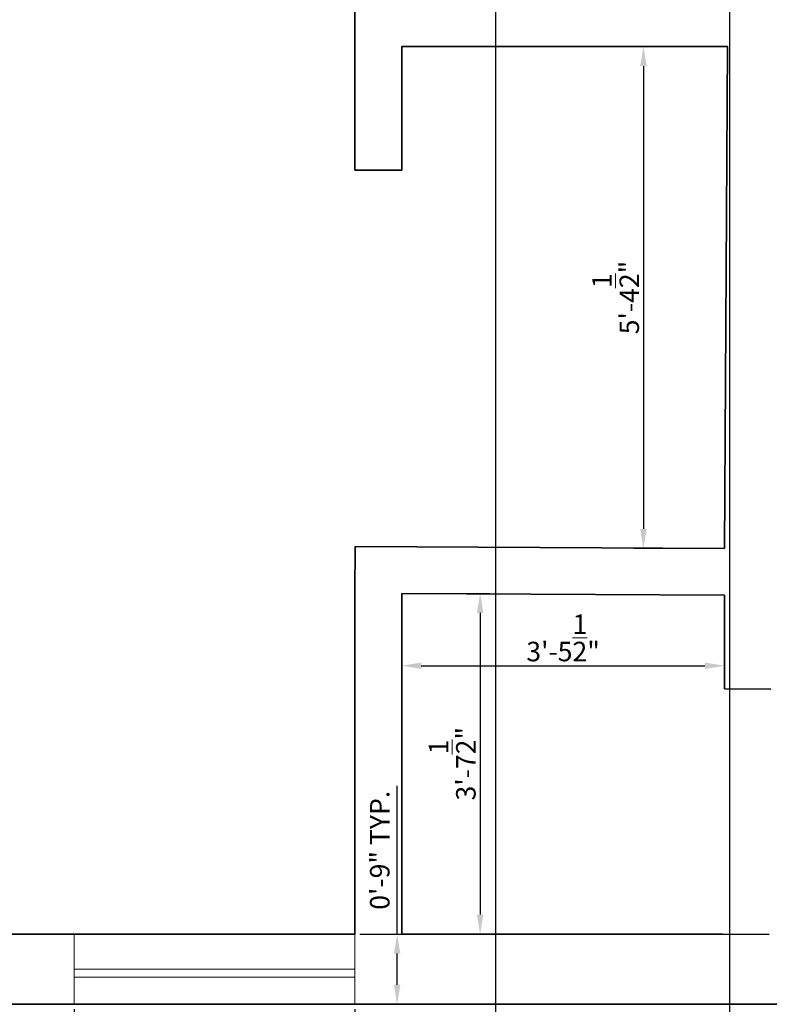
# Model space of a CAD drawing. Units: inches. Extents: x 2025 to 2528, y 1525 to 2336.
# Tile 3 of 18: x 2164 to 2260, y 1704 to 1831. Entities that reach past the tile are written whole.
import ezdxf

# ---------------------------------------------------------------- set-up
doc = ezdxf.new("R2010")
doc.units = ezdxf.units.IN
for name, color, linetype, lineweight in [('A-ANNO-DIMS', 2, 'Continuous', 18), ('A-GLAZ', 4, 'Continuous', 18), ('A-WALL', 7, 'Continuous', 35)]:
    doc.layers.add(name, color=color, linetype=linetype, lineweight=lineweight)
doc.styles.get("Standard").update_dxf_attribs({"font": 'arial.ttf'})
doc.dimstyles.new('Copy of ISO-25', dxfattribs={"dimtxt": 2.5, "dimasz": 2.5, "dimexe": 1.25, "dimexo": 0.625, "dimtad": 1, "dimdec": 1, "dimlunit": 4, "dimtxsty": 'Standard', "dimcen": 2.5, "dimadec": 0, "dimazin": 0, "dimtfac": 1, "dimtdec": 1, "dimtmove": 0, "dimatfit": 3, "dimfxl": 1, "dimarcsym": 0})

# ---------------------------------------------------------------- blocks, each defined once
blk = doc.blocks.new('*D33')
at = {"layer": 'A-ANNO-DIMS', "color": 0, "lineweight": -2, "transparency": 16777216}
for p, q in [((2213.01, 1756.46), (2213.01, 1746.56)), ((2254.35, 1756.23), (2254.35, 1746.56)), ((2215.51, 1747.81), (2251.85, 1747.81))]:
    blk.add_line(p, q, dxfattribs=at)
at = {"layer": 'A-ANNO-DIMS', "color": 0, "transparency": 16777216}
for points in [[(2215.51, 1748.22), (2215.51, 1747.39), (2213.01, 1747.81)], [(2251.85, 1748.22), (2251.85, 1747.39), (2254.35, 1747.81)]]:
    blk.add_solid(points, dxfattribs=at)
at = {"layer": 'Defpoints', "color": 0, "transparency": 16777216}
for p in [(2213.01, 1757.08), (2254.35, 1756.85), (2254.35, 1747.81)]:
    blk.add_point(p, dxfattribs=at)
at = {"layer": 'A-ANNO-DIMS', "color": 0, "transparency": 16777216, "insert": (2233.68, 1751.38), "char_height": 2.5, "attachment_point": 5}
blk.add_mtext('3\'-5{\\H1x;\\S1/2;}"', dxfattribs=at)
blk = doc.blocks.new('*D34')
at = {"layer": 'A-ANNO-DIMS', "color": 0, "lineweight": -2, "transparency": 16777216}
for p, q in [((2213.64, 1757.08), (2224.3, 1757.08)), ((2223.05, 1754.58), (2223.05, 1715.91)), ((2213.64, 1713.41), (2224.3, 1713.41))]:
    blk.add_line(p, q, dxfattribs=at)
at = {"layer": 'A-ANNO-DIMS', "color": 0, "transparency": 16777216}
for points in [[(2222.63, 1754.58), (2223.46, 1754.58), (2223.05, 1757.08)], [(2222.63, 1715.91), (2223.46, 1715.91), (2223.05, 1713.41)]]:
    blk.add_solid(points, dxfattribs=at)
at = {"layer": 'Defpoints', "color": 0, "transparency": 16777216}
for p in [(2213.01, 1757.08), (2213.01, 1713.41), (2223.05, 1713.41)]:
    blk.add_point(p, dxfattribs=at)
at = {"layer": 'A-ANNO-DIMS', "color": 0, "transparency": 16777216, "insert": (2219.47, 1735.25), "char_height": 2.5, "attachment_point": 5, "rotation": 90}
blk.add_mtext('3\'-7{\\H1x;\\S1/2;}"', dxfattribs=at)
blk = doc.blocks.new('*D36')
at = {"layer": 'A-ANNO-DIMS', "color": 0, "lineweight": -2, "transparency": 16777216}
for p, q in [((2254.12, 1827.18), (2242.73, 1827.18)), ((2243.98, 1824.68), (2243.98, 1765.35)), ((2253.76, 1762.85), (2242.73, 1762.85))]:
    blk.add_line(p, q, dxfattribs=at)
at = {"layer": 'A-ANNO-DIMS', "color": 0, "transparency": 16777216}
for points in [[(2243.56, 1824.68), (2244.4, 1824.68), (2243.98, 1827.18)], [(2243.56, 1765.35), (2244.4, 1765.35), (2243.98, 1762.85)]]:
    blk.add_solid(points, dxfattribs=at)
at = {"layer": 'Defpoints', "color": 0, "transparency": 16777216}
for p in [(2254.74, 1827.18), (2243.98, 1762.85), (2254.38, 1762.85)]:
    blk.add_point(p, dxfattribs=at)
at = {"layer": 'A-ANNO-DIMS', "color": 0, "transparency": 16777216, "insert": (2240.41, 1795.01), "char_height": 2.5, "attachment_point": 5, "rotation": 90}
blk.add_mtext('5\'-4{\\H1x;\\S1/2;}"', dxfattribs=at)
blk = doc.blocks.new('WIN-36-PORCH')
for p, q in [((0, 0), (0, 9)), ((36, 9), (36, 0)), ((0, 4.5), (36, 4.5)), ((0, 3.5), (36, 3.5)), ((36, 0), (0, 0))]:
    blk.add_line(p, q)
blk = doc.blocks.new('*D52')
at = {"layer": 'A-ANNO-DIMS', "color": 0, "lineweight": -2, "transparency": 16777216}
for p, q in [((2171.01, 1703.79), (2171.01, 1697.76)), ((2207.01, 1703.79), (2207.01, 1697.76)), ((2173.51, 1699.01), (2204.51, 1699.01))]:
    blk.add_line(p, q, dxfattribs=at)
at = {"layer": 'A-ANNO-DIMS', "color": 0, "transparency": 16777216}
for points in [[(2173.51, 1699.43), (2173.51, 1698.6), (2171.01, 1699.01)], [(2204.51, 1699.43), (2204.51, 1698.6), (2207.01, 1699.01)]]:
    blk.add_solid(points, dxfattribs=at)
at = {"layer": 'Defpoints', "color": 0, "transparency": 16777216}
for p in [(2171.01, 1704.41), (2207.01, 1704.41), (2207.01, 1699.01)]:
    blk.add_point(p, dxfattribs=at)
at = {"layer": 'A-ANNO-DIMS', "color": 0, "transparency": 16777216, "insert": (2189.01, 1700.93), "char_height": 2.5, "attachment_point": 5}
blk.add_mtext('WINDOW 3\'-0" TYP.', dxfattribs=at)
blk = doc.blocks.new('*D53')
at = {"layer": 'A-ANNO-DIMS', "color": 0, "lineweight": -2, "transparency": 16777216}
for p, q in [((2212.41, 1713.41), (2212.41, 1732.4)), ((2207.64, 1713.41), (2213.66, 1713.41)), ((2212.41, 1706.91), (2212.41, 1710.91)), ((2207.64, 1704.41), (2213.66, 1704.41))]:
    blk.add_line(p, q, dxfattribs=at)
at = {"layer": 'A-ANNO-DIMS', "color": 0, "transparency": 16777216}
for points in [[(2212, 1710.91), (2212.83, 1710.91), (2212.41, 1713.41)], [(2212, 1706.91), (2212.83, 1706.91), (2212.41, 1704.41)]]:
    blk.add_solid(points, dxfattribs=at)
at = {"layer": 'Defpoints', "color": 0, "transparency": 16777216}
for p in [(2207.01, 1713.41), (2212.41, 1713.41), (2207.01, 1704.41)]:
    blk.add_point(p, dxfattribs=at)
at = {"layer": 'A-ANNO-DIMS', "color": 0, "transparency": 16777216, "insert": (2210.51, 1724.16), "char_height": 2.5, "attachment_point": 5, "rotation": 90}
blk.add_mtext('0\'-9" TYP.', dxfattribs=at)
blk = doc.blocks.new('*D75')
at = {"layer": 'A-ANNO-DIMS', "color": 0, "lineweight": -2, "transparency": 16777216}
for p, q in [((2225.01, 2114.79), (2225.01, 1525.61)), ((2255.01, 2114.79), (2255.01, 1525.61)), ((2227.51, 1526.86), (2252.51, 1526.86))]:
    blk.add_line(p, q, dxfattribs=at)
at = {"layer": 'A-ANNO-DIMS', "color": 0, "transparency": 16777216}
for points in [[(2227.51, 1527.28), (2227.51, 1526.45), (2225.01, 1526.86)], [(2252.51, 1527.28), (2252.51, 1526.45), (2255.01, 1526.86)]]:
    blk.add_solid(points, dxfattribs=at)
at = {"layer": 'Defpoints', "color": 0, "transparency": 16777216}
for p in [(2225.01, 2115.41), (2255.01, 2115.41), (2255.01, 1526.86)]:
    blk.add_point(p, dxfattribs=at)
at = {"layer": 'A-ANNO-DIMS', "color": 0, "transparency": 16777216, "insert": (2240.01, 1528.76), "char_height": 2.5, "attachment_point": 5}
blk.add_mtext('2\'-6"', dxfattribs=at)
blk = doc.blocks.new('*D80')
at = {"layer": 'A-ANNO-DIMS', "color": 0, "lineweight": -2, "transparency": 16777216}
for p, q in [((2065.39, 2292.41), (2027.21, 2292.41)), ((2028.46, 1566.91), (2028.46, 2289.91)), ((2285.39, 1564.41), (2027.21, 1564.41))]:
    blk.add_line(p, q, dxfattribs=at)
at = {"layer": 'A-ANNO-DIMS', "color": 0, "transparency": 16777216}
for points in [[(2028.05, 2289.91), (2028.88, 2289.91), (2028.46, 2292.41)], [(2028.05, 1566.91), (2028.88, 1566.91), (2028.46, 1564.41)]]:
    blk.add_solid(points, dxfattribs=at)
at = {"layer": 'Defpoints', "color": 0, "transparency": 16777216}
for p in [(2028.46, 2292.41), (2066.01, 2292.41), (2286.01, 1564.41)]:
    blk.add_point(p, dxfattribs=at)
at = {"layer": 'A-ANNO-DIMS', "color": 0, "transparency": 16777216, "insert": (2026.56, 1928.41), "char_height": 2.5, "attachment_point": 5, "rotation": 90}
blk.add_mtext('60\'-8"', dxfattribs=at)

msp = doc.modelspace()

# ---------------------------------------------------------------- linework, layer by layer
at = {"layer": 'A-WALL'}
for p, q in [((2207.01, 1827.18), (2207.01, 1869.41)), ((2207.01, 1827.18), (2207.01, 1811.35)), ((2254.78, 1827.18), (2213.01, 1827.18)), ((2213.01, 1811.35), (2213.01, 1827.18)), ((2254.74, 1827.18), (2254.38, 1762.85)), ((2207.01, 1811.35), (2213.01, 1811.35)), ((2207.05, 1763.11), (2207.01, 1757.12)), ((2207.05, 1763.11), (2254.38, 1762.85)), ((2207.01, 1757.12), (2207.01, 1713.41)), ((2207.01, 1713.41), (2207.01, 1757.12)), ((2213.01, 1757.08), (2213.01, 1713.41)), ((2213.01, 1757.08), (2254.35, 1756.85)), ((2254.35, 1756.85), (2254.35, 1744.85)), ((2254.35, 1744.85), (2260.29, 1744.82)), ((2075.01, 1713.41), (2207.01, 1713.41)), ((2171.01, 1713.41), (2135.01, 1713.41)), ((2213.01, 1713.41), (2254.11, 1713.41)), ((2254.11, 1713.41), (2260.11, 1713.38)), ((2066.01, 1704.41), (2489.01, 1704.41))]:
    msp.add_line(p, q, dxfattribs=at)

# ---------------------------------------------------------------- block references
at = {"layer": 'A-GLAZ'}
msp.add_blockref('WIN-36-PORCH', (2171.01, 1704.41), dxfattribs=at)

# ---------------------------------------------------------------- dimensions: what is measured, and where the dimension line sits
at = {"layer": 'A-ANNO-DIMS'}
for base, p1, p2, override, picture, middle in [((2028.46, 2292.41), (2286.01, 1564.41), (2066.01, 2292.41), {"dimdec": 1, "dimlfac": 1, "dimrnd": 0, "dimzin": 1, "dimdsep": 46, "dimlunit": 4, "dimfrac": 2}, '*D80', (2026.56, 1928.41)), ((2243.98, 1762.85), (2254.74, 1827.18), (2254.38, 1762.85), {"dimclrd": 0, "dimclre": 0, "dimclrt": 0}, '*D36', (2240.41, 1795.01)), ((2223.05, 1713.41), (2213.01, 1757.08), (2213.01, 1713.41), {"dimclrd": 0, "dimclre": 0, "dimclrt": 0}, '*D34', (2219.47, 1735.25))]:
    dim = msp.add_linear_dim(base=base, p1=p1, p2=p2, angle=90, dimstyle='Copy of ISO-25', override=override, dxfattribs=at)
    dim.commit()
    dim.dimension.update_dxf_attribs({"geometry": picture, "text_midpoint": middle})
for base, p1, p2, override, picture, middle in [((2255.01, 1526.86), (2225.01, 2115.41), (2255.01, 2115.41), {"dimdec": 1, "dimlfac": 1, "dimrnd": 0, "dimzin": 1, "dimdsep": 46, "dimlunit": 4, "dimfrac": 2}, '*D75', (2240.01, 1528.76)), ((2254.35, 1747.81), (2213.01, 1757.08), (2254.35, 1756.85), {"dimclrd": 0, "dimclre": 0, "dimclrt": 0}, '*D33', (2233.68, 1751.38))]:
    dim = msp.add_linear_dim(base=base, p1=p1, p2=p2, dimstyle='Copy of ISO-25', override=override, dxfattribs=at)
    dim.commit()
    dim.dimension.update_dxf_attribs({"geometry": picture, "text_midpoint": middle})
dim = msp.add_linear_dim(base=(2212.41, 1713.41), p1=(2207.01, 1704.41), p2=(2207.01, 1713.41), angle=90, text='<> TYP.', dimstyle='Copy of ISO-25', override={"dimdec": 1, "dimlfac": 1, "dimrnd": 0, "dimzin": 1, "dimdsep": 46, "dimlunit": 4, "dimfrac": 2}, dxfattribs=at)
dim.commit()
dim.dimension.update_dxf_attribs({"geometry": '*D53', "text_midpoint": (2210.51, 1724.16)})
dim = msp.add_linear_dim(base=(2207.01, 1699.01), p1=(2171.01, 1704.41), p2=(2207.01, 1704.41), text='WINDOW <> TYP.', dimstyle='Copy of ISO-25', override={"dimdec": 1, "dimlfac": 1, "dimrnd": 0, "dimzin": 1, "dimdsep": 46, "dimlunit": 4, "dimfrac": 2}, dxfattribs=at)
dim.commit()
dim.dimension.update_dxf_attribs({"geometry": '*D52', "text_midpoint": (2189.01, 1700.93)})

doc.saveas('drawing.dxf')
